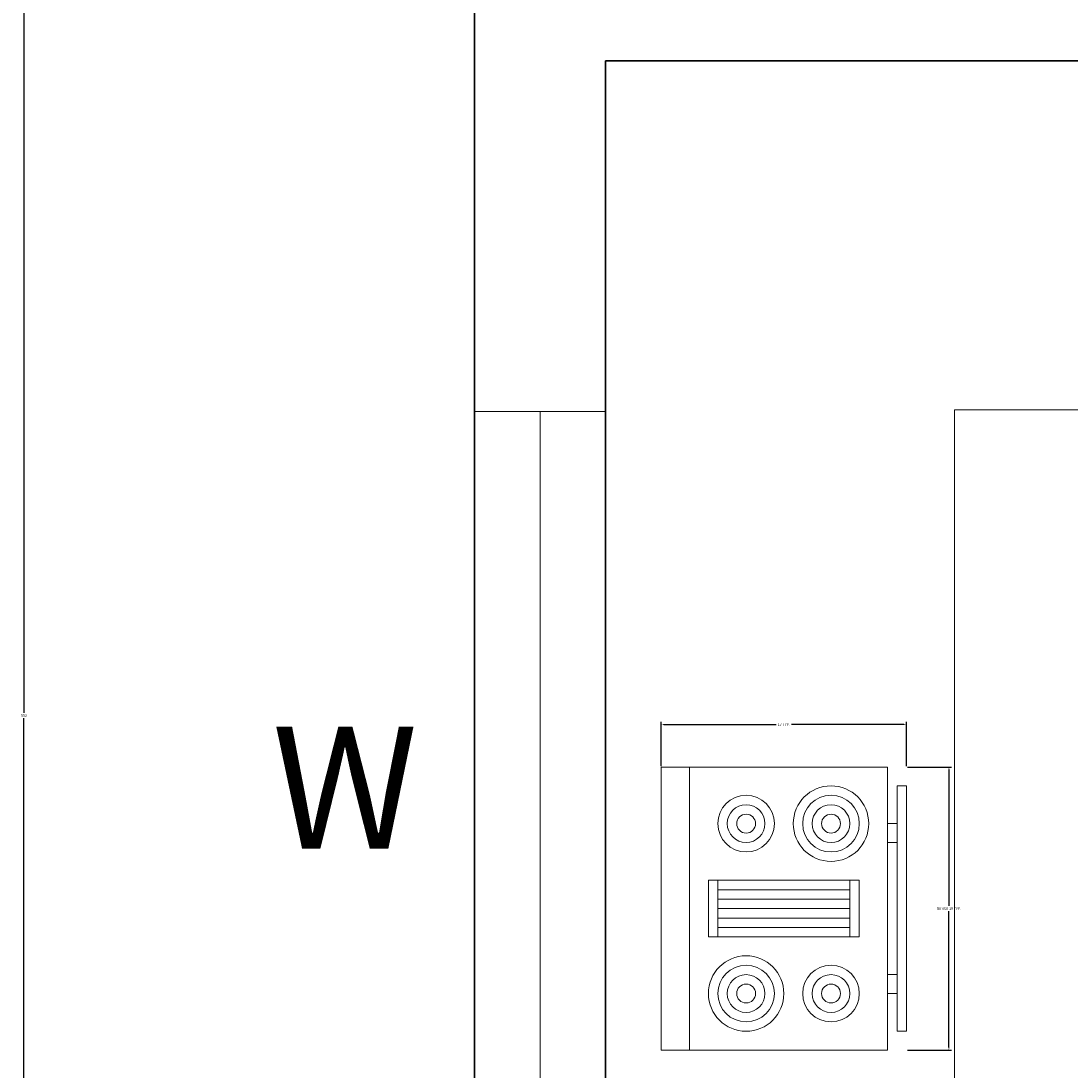
# Model space of a CAD drawing. Units: feet. Extents: x 1654 to 2985, y 1348 to 2230.
# Tile 6 of 53: x 1812 to 1884, y 1817 to 1889. Entities that reach past the tile are written whole.
import ezdxf

# ---------------------------------------------------------------- set-up
doc = ezdxf.new("R2010")
doc.units = ezdxf.units.FT
for name, color, linetype, lineweight in [('A-ANNO-DIMS', 2, 'Continuous', 18), ('A-ANNO-TEXT', 7, 'Continuous', 18), ('A-EQPM', 9, 'Continuous', 18), ('A-FLOR-CASE', 8, 'Continuous', 18), ('A-GLAZ', 4, 'Continuous', 18), ('A-WALL', 7, 'Continuous', 35)]:
    doc.layers.add(name, color=color, linetype=linetype, lineweight=lineweight)
doc.styles.get("Standard").update_dxf_attribs({"font": 'arial.ttf'})
doc.dimstyles.get("Standard").update_dxf_attribs({"dimtxt": 0.18, "dimasz": 0.18, "dimexe": 0.18, "dimexo": 0.0625, "dimgap": 0.09, "dimtad": 0, "dimtih": 1, "dimtoh": 1, "dimdec": 4, "dimzin": 0, "dimdsep": 46, "dimtxsty": 'Standard', "dimcen": 0.09, "dimadec": 0, "dimazin": 0, "dimtfac": 1, "dimtdec": 4, "dimtofl": 0, "dimtmove": 0, "dimatfit": 3, "dimfxl": 1, "dimtolj": 1, "dimtzin": 0, "dimarcsym": 0})

# ---------------------------------------------------------------- blocks, each defined once
blk = doc.blocks.new('Range-Oven - 30 in top')
for p, q in [((0, -3), (30, -3)), ((12, -6), (18, -6)), ((13, -20), (13, -6)), ((14, -6), (14, -20)), ((15, -20), (15, -6)), ((16, -6), (16, -20)), ((17, -20), (17, -6)), ((18, -20), (12, -20)), ((6, -24), (6, -25)), ((8, -25), (8, -24)), ((22, -25), (22, -24)), ((24, -24), (24, -25))]:
    blk.add_line(p, q)
for points in [[(0, -24), (0, 0), (30, 0), (30, -24)], [(12, -21), (12, -5), (18, -5), (18, -21)], [(2, -26), (2, -25), (28, -25), (28, -26)]]:
    blk.add_lwpolyline(points, close=True)
for centre, radius in [((6, -9), 4), ((6, -9), 3), ((24, -9), 3), ((6, -9), 2), ((24, -9), 2), ((6, -9), 1), ((24, -9), 1), ((24, -18), 4), ((6, -18), 3), ((24, -18), 3), ((6, -18), 2), ((24, -18), 2), ((6, -18), 1), ((24, -18), 1)]:
    blk.add_circle(centre, radius)
blk = doc.blocks.new('WIN-KITCHEN')
for p, q in [((0, 60.691), (9, 60.691)), ((4.5, 60.691), (4.5, 0)), ((0, 0), (9, 0))]:
    blk.add_line(p, q)
blk = doc.blocks.new('CASEWORK-KITCHEN-L')
for q in [(72, 111), (0, 0)]:
    blk.add_line((0, 111), q)
blk = doc.blocks.new('*D44')
at = {"layer": 'A-ANNO-DIMS', "color": 0, "lineweight": -2, "transparency": 16777216}
for p, q in [((1872.858, 1837.712), (1875.896, 1837.712)), ((1875.716, 1837.532), (1875.716, 1828.162)), ((1875.716, 1818.426), (1875.716, 1827.796)), ((1872.858, 1818.246), (1875.896, 1818.246))]:
    blk.add_line(p, q, dxfattribs=at)
at = {"layer": 'A-ANNO-DIMS', "color": 0, "transparency": 16777216}
for points in [[(1875.686, 1837.532), (1875.746, 1837.532), (1875.716, 1837.712)], [(1875.686, 1818.426), (1875.746, 1818.426), (1875.716, 1818.246)]]:
    blk.add_solid(points, dxfattribs=at)
at = {"layer": 'Defpoints', "color": 0, "transparency": 16777216}
for p in [(1872.796, 1837.712), (1875.716, 1837.712), (1872.796, 1818.246)]:
    blk.add_point(p, dxfattribs=at)
at = {"layer": 'A-ANNO-DIMS', "color": 0, "transparency": 16777216, "insert": (1875.716, 1827.979), "char_height": 0.18, "attachment_point": 5}
blk.add_mtext('\\A1;RANGE 19 TYP.', dxfattribs=at)
blk = doc.blocks.new('*D45')
at = {"layer": 'A-ANNO-DIMS', "color": 0, "lineweight": -2, "transparency": 16777216}
for p, q in [((1855.925, 1837.775), (1855.925, 1840.812)), ((1856.105, 1840.632), (1863.841, 1840.632)), ((1872.616, 1840.632), (1864.88, 1840.632)), ((1872.796, 1837.775), (1872.796, 1840.812))]:
    blk.add_line(p, q, dxfattribs=at)
at = {"layer": 'A-ANNO-DIMS', "color": 0, "transparency": 16777216}
for points in [[(1856.105, 1840.662), (1856.105, 1840.602), (1855.925, 1840.632)], [(1872.616, 1840.662), (1872.616, 1840.602), (1872.796, 1840.632)]]:
    blk.add_solid(points, dxfattribs=at)
at = {"layer": 'Defpoints', "color": 0, "transparency": 16777216}
for p in [(1855.925, 1840.632), (1855.925, 1837.712), (1872.796, 1837.712)]:
    blk.add_point(p, dxfattribs=at)
at = {"layer": 'A-ANNO-DIMS', "color": 0, "transparency": 16777216, "insert": (1864.36, 1840.632), "char_height": 0.18, "attachment_point": 5}
blk.add_mtext('\\A1;17 TYP.', dxfattribs=at)
blk = doc.blocks.new('*D77')
at = {"layer": 'A-ANNO-DIMS', "color": 0, "lineweight": -2, "transparency": 16777216}
for p, q in [((1843.03, 2117.255), (1811.912, 2117.255)), ((1812.092, 2117.075), (1812.092, 1841.437)), ((1812.092, 1565.435), (1812.092, 1841.073)), ((1843.03, 1565.255), (1811.912, 1565.255))]:
    blk.add_line(p, q, dxfattribs=at)
at = {"layer": 'A-ANNO-DIMS', "color": 0, "transparency": 16777216}
for points in [[(1812.062, 2117.075), (1812.122, 2117.075), (1812.092, 2117.255)], [(1812.062, 1565.435), (1812.122, 1565.435), (1812.092, 1565.255)]]:
    blk.add_solid(points, dxfattribs=at)
at = {"layer": 'Defpoints', "color": 0, "transparency": 16777216}
for p in [(1812.092, 2117.255), (1843.092, 2117.255), (1843.092, 1565.255)]:
    blk.add_point(p, dxfattribs=at)
at = {"layer": 'A-ANNO-DIMS', "color": 0, "transparency": 16777216, "insert": (1812.092, 1841.255), "char_height": 0.18, "attachment_point": 5}
blk.add_mtext('\\A1;552', dxfattribs=at)

msp = doc.modelspace()

# ---------------------------------------------------------------- linework, layer by layer
at = {"layer": 'A-WALL'}
for p, q in [((1843.0924, 2117.2549), (1843.0924, 1565.2549)), ((1843.0924, 1886.2549), (1843.0924, 1751.2549)), ((1852.0924, 1886.2549), (1948.0924, 1886.2549)), ((1852.0924, 1886.2549), (1852.0924, 1751.2549))]:
    msp.add_line(p, q, dxfattribs=at)

# ---------------------------------------------------------------- block references
at = {"layer": 'A-EQPM', "xscale": 0.6488816563275249, "yscale": 0.6488816563275249, "zscale": 0.6488816563275249, "rotation": 90}
msp.add_blockref('Range-Oven - 30 in top', (1855.9248, 1818.2456), dxfattribs=at)
at = {"layer": 'A-FLOR-CASE'}
msp.add_blockref('CASEWORK-KITCHEN-L', (1876.092, 1751.255), dxfattribs=at)
at = {"layer": 'A-GLAZ'}
msp.add_blockref('WIN-KITCHEN', (1843.092, 1801.468), dxfattribs=at)

# ---------------------------------------------------------------- texts
at = {"layer": 'A-ANNO-TEXT'}
msp.add_text('W', height=8.3811, dxfattribs=at).set_placement((1829.1535, 1832.0964))

# ---------------------------------------------------------------- dimensions: what is measured, and where the dimension line sits
at = {"layer": 'A-ANNO-DIMS'}
dim = msp.add_linear_dim(base=(1812.0924, 2117.2549), p1=(1843.0924, 1565.2549), p2=(1843.0924, 2117.2549), angle=90, dimstyle='Standard', override={"dimdec": 0, "dimlfac": 1, "dimrnd": 0, "dimzin": 0, "dimdsep": 46, "dimlunit": 2}, dxfattribs=at)
dim.commit()
dim.dimension.update_dxf_attribs({"geometry": '*D77', "text_midpoint": (1812.0924, 1841.2549)})
for base, p1, p2, angle, text, picture, middle in [((1855.9248, 1840.632), (1872.7958, 1837.712), (1855.9248, 1837.712), 180, '<> TYP.', '*D45', (1864.3603, 1840.632)), ((1875.7157, 1837.712), (1872.7958, 1818.2456), (1872.7958, 1837.712), 90, 'RANGE <> TYP.', '*D44', (1875.7157, 1827.9788))]:
    dim = msp.add_linear_dim(base=base, p1=p1, p2=p2, angle=angle, text=text, dimstyle='Standard', override={"dimdec": 0, "dimlfac": 1, "dimrnd": 0, "dimzin": 0, "dimdsep": 46, "dimlunit": 2}, dxfattribs=at)
    dim.commit()
    dim.dimension.update_dxf_attribs({"geometry": picture, "text_midpoint": middle})

doc.saveas('drawing.dxf')
